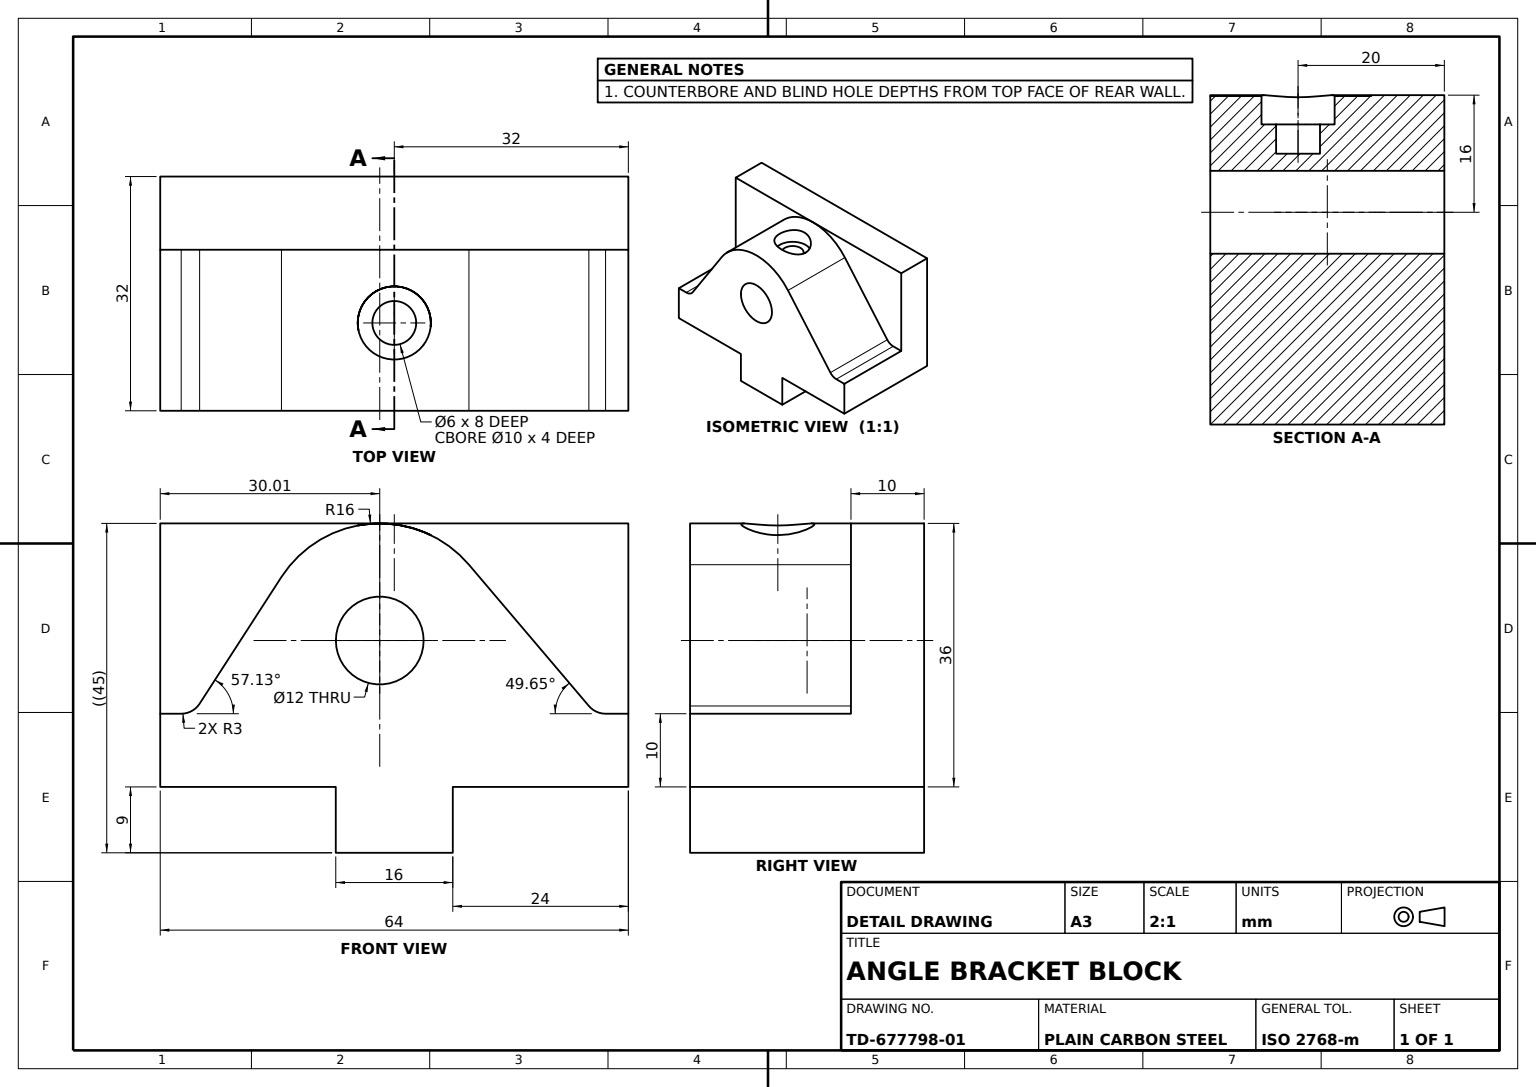
SolidWorks part; units mm, degrees
material "Plain Carbon Steel"
ref_plane "Front Plane" through (0, 0, 0) normal (0, 0, 1) x (1, 0, 0)
ref_plane "Top Plane" through (0, 0, 0) normal (0, 1, 0) x (1, 0, 0)
ref_plane "Right Plane" through (0, 0, 0) normal (1, 0, 0) x (0, 0, -1)
sketch "Jaw Body Profile Sketch" plane through (0, 0, 0) normal (0, 0, 1) x (1, 0, 0)
  line L0 (0, 0) -> (32, 0)
  line L1 (32, 0) -> (32, 10)
  line L2 (32, 10) -> (10, 10)
  line L3 (10, 10) -> (10, 36)
  line L4 (10, 36) -> (0, 36)
  line L5 (0, 36) -> (0, 0)
  dimension "D1" = 36
  dimension "D2" = 32
  dimension "D3" = 10
  dimension "D4" = 10
extrude "Jaw Body" add sketch "Jaw Body Profile Sketch" against normal blind 64
sketch "Pivot Boss Sketch" plane through (32, 0, 0) normal (1, 0, 0) x (0, 0, -1)
  line L0 (4.5, 10) -> (16.5742, 28.6841)
  line L1 (64, 10) -> (0, 10) construction
  line L2 (42.2068, 30.3584) -> (59.5, 10)
  line L3 (64, 10) -> (0, 10) construction
  line L4 (64, 36) -> (0, 36) construction
  line L5 (4.5, 10) -> (59.5, 10)
  arc A0 (16.5742, 28.6841) -> (42.2068, 30.3584) centre (30.0124, 20) cw
  dimension "D1" = 16
  dimension "D2" = 55
  dimension "D3" = 4.5
  dimension "D4" = 12.0742
extrude "Pivot Boss" add sketch "Pivot Boss Sketch" against normal up to surface (22 mm away) up to face at (10, 23, -32)
sketch "Pivot Bore Sketch" plane through (32, 0, 0) normal (1, 0, 0) x (0, 0, -1)
  circle A0 centre (30.0124, 20) radius 6
  dimension "D1" = 12
extrude "Pivot Bore Ø12" cut sketch "Pivot Bore Sketch" against normal up to surface (32 mm away) up to face at (0, 18, -32)
sketch "Guide Key Sketch" plane through (32, 0, 0) normal (1, 0, 0) x (0, 0, -1)
  line L1 (64, 0) -> (0, 0) construction
  line L2 (24, 0) -> (40, 0)
  line L3 (24, 0) -> (24, -9)
  line L4 (24, -9) -> (40, -9)
  line L5 (40, 0) -> (40, -9)
  dimension "D1" = 16
  dimension "D2" = 24
  dimension "D3" = 9
extrude "Guide Key" add sketch "Guide Key Sketch" against normal up to surface (32 mm away) up to face at (0, 20, -24.0124)
fillet "Pivot Boss Fillet R3" radius 3 2 edges at (21, 10, -59.5) (21, 10, -4.5)
sketch "Counterbore Sketch" plane through (0, 36, 0) normal (0, 1, 0) x (1, 0, 0)
  line L0 (0, 64) -> (0, 0) construction
  circle A0 centre (20, 32) radius 5
  dimension "D3" = 10
  dimension "D1" = 32
  dimension "D2" = 20
extrude "Counterbore Ø10x4" cut sketch "Counterbore Sketch" against normal blind 4
sketch "Screw Hole Sketch" plane through (0, 32, 0) normal (0, 1, 0) x (1, 0, 0)
  circle A0 centre (20, 32) radius 3
  dimension "D1" = 6
extrude "Screw Hole Ø6x4" cut sketch "Screw Hole Sketch" against normal blind 4
